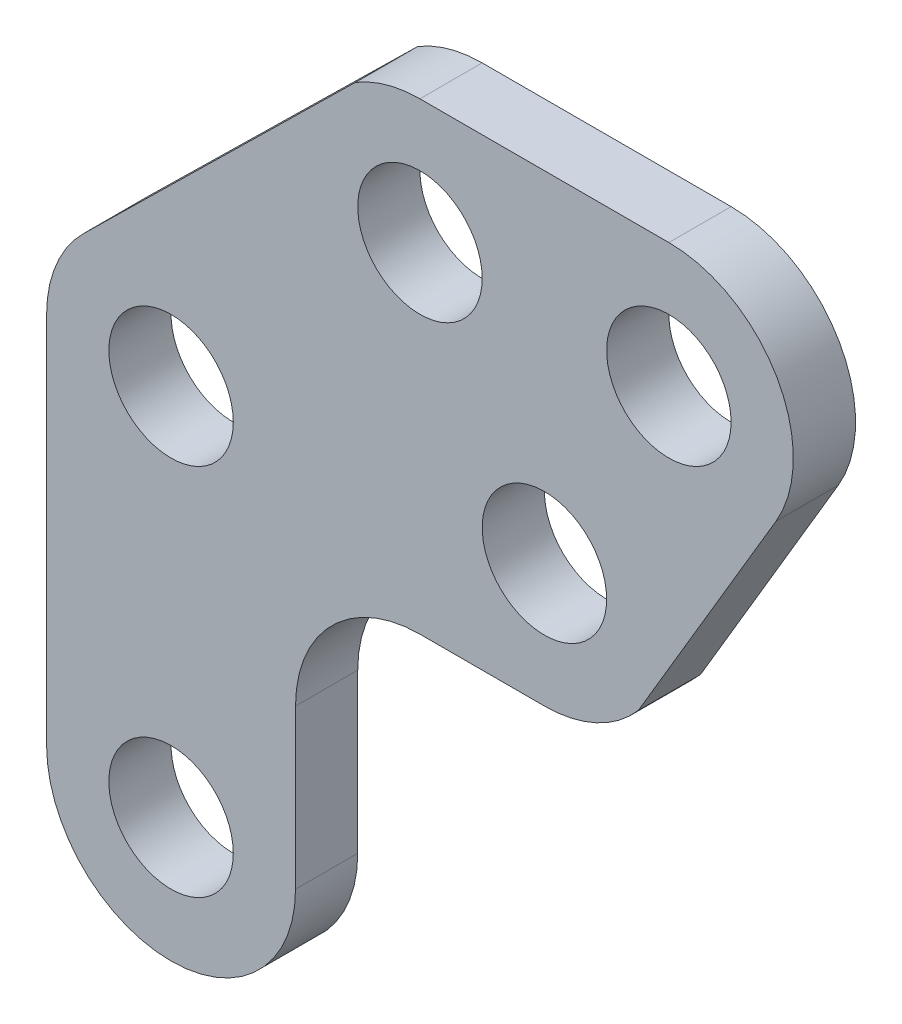
ISO-10303-21;
HEADER;
FILE_DESCRIPTION(('STEP AP214'),'2;1');
FILE_NAME('part.step','',(''),(''),'','','');
FILE_SCHEMA(('AUTOMOTIVE_DESIGN { 1 0 10303 214 1 1 1 1 }'));
ENDSEC;
DATA;
#1=APPLICATION_CONTEXT('core data for automotive mechanical design processes');
#2=APPLICATION_PROTOCOL_DEFINITION('international standard','automotive_design',2000,#1);
#3=PRODUCT_CONTEXT('',#1,'mechanical');
#4=PRODUCT('Part','Part','',(#3));
#5=PRODUCT_RELATED_PRODUCT_CATEGORY('part','',(#4));
#6=PRODUCT_DEFINITION_FORMATION('','',#4);
#7=PRODUCT_DEFINITION_CONTEXT('part definition',#1,'design');
#8=PRODUCT_DEFINITION('design','',#6,#7);
#9=PRODUCT_DEFINITION_SHAPE('','',#8);
#10=(LENGTH_UNIT() NAMED_UNIT(*) SI_UNIT(.MILLI.,.METRE.));
#11=(NAMED_UNIT(*) PLANE_ANGLE_UNIT() SI_UNIT($,.RADIAN.));
#12=(NAMED_UNIT(*) SI_UNIT($,.STERADIAN.) SOLID_ANGLE_UNIT());
#13=UNCERTAINTY_MEASURE_WITH_UNIT(LENGTH_MEASURE(1.E-05),#10,'distance_accuracy_value','');
#14=(GEOMETRIC_REPRESENTATION_CONTEXT(3) GLOBAL_UNCERTAINTY_ASSIGNED_CONTEXT((#13)) GLOBAL_UNIT_ASSIGNED_CONTEXT((#10,
#11,#12)) REPRESENTATION_CONTEXT('',''));
#15=CARTESIAN_POINT('',(0.,0.,0.));
#16=DIRECTION('',(0.,0.,1.));
#17=DIRECTION('',(1.,0.,0.));
#18=AXIS2_PLACEMENT_3D('',#15,#16,#17);
#19=CARTESIAN_POINT('',(0.,12.7,-3.175));
#20=DIRECTION('',(0.,0.,1.));
#21=DIRECTION('',(1.,0.,0.));
#22=AXIS2_PLACEMENT_3D('',#19,#20,#21);
#23=CYLINDRICAL_SURFACE('',#22,6.35);
#24=CARTESIAN_POINT('',(0.,12.7,0.));
#25=DIRECTION('',(0.,0.,1.));
#26=DIRECTION('',(1.,0.,0.));
#27=AXIS2_PLACEMENT_3D('',#24,#25,#26);
#28=CIRCLE('',#27,6.35);
#29=CARTESIAN_POINT('',(0.,19.05,0.));
#30=VERTEX_POINT('',#29);
#31=CARTESIAN_POINT('',(-3.29150229370883,18.1303326463956,0.));
#32=VERTEX_POINT('',#31);
#33=EDGE_CURVE('E163',#30,#32,#28,.T.);
#34=ORIENTED_EDGE('',*,*,#33,.F.);
#35=DIRECTION('',(0.,0.,1.));
#36=VECTOR('',#35,1.);
#37=CARTESIAN_POINT('',(0.,19.05,-3.175));
#38=LINE('',#37,#36);
#39=CARTESIAN_POINT('',(0.,19.05,-3.175));
#40=VERTEX_POINT('',#39);
#41=EDGE_CURVE('E11',#40,#30,#38,.T.);
#42=ORIENTED_EDGE('',*,*,#41,.F.);
#43=CARTESIAN_POINT('',(0.,12.7,-3.175));
#44=DIRECTION('',(0.,0.,1.));
#45=DIRECTION('',(1.,0.,0.));
#46=AXIS2_PLACEMENT_3D('',#43,#44,#45);
#47=CIRCLE('',#46,6.35);
#48=CARTESIAN_POINT('',(-3.29150229370883,18.1303326463956,-3.175));
#49=VERTEX_POINT('',#48);
#50=EDGE_CURVE('E197',#40,#49,#47,.T.);
#51=ORIENTED_EDGE('',*,*,#50,.T.);
#52=DIRECTION('',(0.,0.,1.));
#53=VECTOR('',#52,1.);
#54=CARTESIAN_POINT('',(-3.29150229370883,18.1303326463956,-3.175));
#55=LINE('',#54,#53);
#56=EDGE_CURVE('E46',#49,#32,#55,.T.);
#57=ORIENTED_EDGE('',*,*,#56,.T.);
#58=EDGE_LOOP('',(#34,#42,#51,#57));
#59=FACE_BOUND('',#58,.T.);
#60=ADVANCED_FACE('F43',(#59),#23,.T.);
#61=CARTESIAN_POINT('',(0.,19.05,-3.175));
#62=DIRECTION('',(0.,1.,0.));
#63=DIRECTION('',(0.,0.,1.));
#64=AXIS2_PLACEMENT_3D('',#61,#62,#63);
#65=PLANE('',#64);
#66=DIRECTION('',(-1.,0.,0.));
#67=VECTOR('',#66,1.);
#68=CARTESIAN_POINT('',(0.,19.05,0.));
#69=LINE('',#68,#67);
#70=CARTESIAN_POINT('',(12.7,19.05,0.));
#71=VERTEX_POINT('',#70);
#72=EDGE_CURVE('E191',#71,#30,#69,.T.);
#73=ORIENTED_EDGE('',*,*,#72,.F.);
#74=DIRECTION('',(0.,0.,1.));
#75=VECTOR('',#74,1.);
#76=CARTESIAN_POINT('',(12.7,19.05,-3.175));
#77=LINE('',#76,#75);
#78=CARTESIAN_POINT('',(12.7,19.05,-3.175));
#79=VERTEX_POINT('',#78);
#80=EDGE_CURVE('E55',#79,#71,#77,.T.);
#81=ORIENTED_EDGE('',*,*,#80,.F.);
#82=DIRECTION('',(-1.,0.,0.));
#83=VECTOR('',#82,1.);
#84=CARTESIAN_POINT('',(0.,19.05,-3.175));
#85=LINE('',#84,#83);
#86=EDGE_CURVE('E152',#79,#40,#85,.T.);
#87=ORIENTED_EDGE('',*,*,#86,.T.);
#88=ORIENTED_EDGE('',*,*,#41,.T.);
#89=EDGE_LOOP('',(#73,#81,#87,#88));
#90=FACE_BOUND('',#89,.T.);
#91=ADVANCED_FACE('F220',(#90),#65,.T.);
#92=CARTESIAN_POINT('',(12.7,12.7,-3.175));
#93=DIRECTION('',(0.,0.,1.));
#94=DIRECTION('',(1.,0.,0.));
#95=AXIS2_PLACEMENT_3D('',#92,#93,#94);
#96=CYLINDRICAL_SURFACE('',#95,6.35);
#97=CARTESIAN_POINT('',(12.7,12.7,0.));
#98=DIRECTION('',(0.,0.,1.));
#99=DIRECTION('',(1.,0.,0.));
#100=AXIS2_PLACEMENT_3D('',#97,#98,#99);
#101=CIRCLE('',#100,6.35);
#102=CARTESIAN_POINT('',(18.1648692173738,9.46616258340034,0.));
#103=VERTEX_POINT('',#102);
#104=EDGE_CURVE('E143',#103,#71,#101,.T.);
#105=ORIENTED_EDGE('',*,*,#104,.F.);
#106=DIRECTION('',(0.,0.,1.));
#107=VECTOR('',#106,1.);
#108=CARTESIAN_POINT('',(18.1648692173738,9.46616258340034,-3.175));
#109=LINE('',#108,#107);
#110=CARTESIAN_POINT('',(18.1648692173738,9.46616258340034,-3.175));
#111=VERTEX_POINT('',#110);
#112=EDGE_CURVE('E137',#111,#103,#109,.T.);
#113=ORIENTED_EDGE('',*,*,#112,.F.);
#114=CARTESIAN_POINT('',(12.7,12.7,-3.175));
#115=DIRECTION('',(0.,0.,1.));
#116=DIRECTION('',(1.,0.,0.));
#117=AXIS2_PLACEMENT_3D('',#114,#115,#116);
#118=CIRCLE('',#117,6.35);
#119=EDGE_CURVE('E139',#111,#79,#118,.T.);
#120=ORIENTED_EDGE('',*,*,#119,.T.);
#121=ORIENTED_EDGE('',*,*,#80,.T.);
#122=EDGE_LOOP('',(#105,#113,#120,#121));
#123=FACE_BOUND('',#122,.T.);
#124=ADVANCED_FACE('F138',(#123),#96,.T.);
#125=CARTESIAN_POINT('',(11.1439713813353,-2.39846866415228,-3.175));
#126=DIRECTION('',(0.86060932557068,-0.509265734897587,0.));
#127=DIRECTION('',(0.509265734897587,0.86060932557068,0.));
#128=AXIS2_PLACEMENT_3D('',#125,#126,#127);
#129=PLANE('',#128);
#130=DIRECTION('',(0.509265734897587,0.86060932557068,0.));
#131=VECTOR('',#130,1.);
#132=CARTESIAN_POINT('',(11.1439713813353,-2.39846866415228,0.));
#133=LINE('',#132,#131);
#134=CARTESIAN_POINT('',(11.1439713813353,-2.39846866415228,0.));
#135=VERTEX_POINT('',#134);
#136=EDGE_CURVE('E195',#135,#103,#133,.T.);
#137=ORIENTED_EDGE('',*,*,#136,.F.);
#138=DIRECTION('',(0.,0.,1.));
#139=VECTOR('',#138,1.);
#140=CARTESIAN_POINT('',(11.1439713813353,-2.39846866415228,-3.175));
#141=LINE('',#140,#139);
#142=CARTESIAN_POINT('',(11.1439713813353,-2.39846866415228,-3.175));
#143=VERTEX_POINT('',#142);
#144=EDGE_CURVE('E148',#143,#135,#141,.T.);
#145=ORIENTED_EDGE('',*,*,#144,.F.);
#146=DIRECTION('',(0.509265734897587,0.86060932557068,0.));
#147=VECTOR('',#146,1.);
#148=CARTESIAN_POINT('',(11.1439713813353,-2.39846866415228,-3.175));
#149=LINE('',#148,#147);
#150=EDGE_CURVE('E155',#143,#111,#149,.T.);
#151=ORIENTED_EDGE('',*,*,#150,.T.);
#152=ORIENTED_EDGE('',*,*,#112,.T.);
#153=EDGE_LOOP('',(#137,#145,#151,#152));
#154=FACE_BOUND('',#153,.T.);
#155=ADVANCED_FACE('F156',(#154),#129,.T.);
#156=CARTESIAN_POINT('',(6.34999999999995,1.70147737193766,-3.175));
#157=DIRECTION('',(0.,0.,1.));
#158=DIRECTION('',(1.,0.,0.));
#159=AXIS2_PLACEMENT_3D('',#156,#157,#158);
#160=CYLINDRICAL_SURFACE('',#159,6.30806777895673);
#161=CARTESIAN_POINT('',(6.34999999999995,1.70147737193766,0.));
#162=DIRECTION('',(0.,0.,1.));
#163=DIRECTION('',(1.,0.,0.));
#164=AXIS2_PLACEMENT_3D('',#161,#162,#163);
#165=CIRCLE('',#164,6.30806777895673);
#166=CARTESIAN_POINT('',(6.34999999999995,-4.60659040701907,0.));
#167=VERTEX_POINT('',#166);
#168=EDGE_CURVE('E188',#167,#135,#165,.T.);
#169=ORIENTED_EDGE('',*,*,#168,.F.);
#170=DIRECTION('',(0.,0.,1.));
#171=VECTOR('',#170,1.);
#172=CARTESIAN_POINT('',(6.34999999999995,-4.60659040701907,-3.175));
#173=LINE('',#172,#171);
#174=CARTESIAN_POINT('',(6.34999999999995,-4.60659040701907,-3.175));
#175=VERTEX_POINT('',#174);
#176=EDGE_CURVE('E203',#175,#167,#173,.T.);
#177=ORIENTED_EDGE('',*,*,#176,.F.);
#178=CARTESIAN_POINT('',(6.34999999999995,1.70147737193766,-3.175));
#179=DIRECTION('',(0.,0.,1.));
#180=DIRECTION('',(1.,0.,0.));
#181=AXIS2_PLACEMENT_3D('',#178,#179,#180);
#182=CIRCLE('',#181,6.30806777895673);
#183=EDGE_CURVE('E160',#175,#143,#182,.T.);
#184=ORIENTED_EDGE('',*,*,#183,.T.);
#185=ORIENTED_EDGE('',*,*,#144,.T.);
#186=EDGE_LOOP('',(#169,#177,#184,#185));
#187=FACE_BOUND('',#186,.T.);
#188=ADVANCED_FACE('F229',(#187),#160,.T.);
#189=CARTESIAN_POINT('',(6.34999999999995,-4.60659040701907,-3.175));
#190=DIRECTION('',(0.,-1.,0.));
#191=DIRECTION('',(1.,0.,0.));
#192=AXIS2_PLACEMENT_3D('',#189,#190,#191);
#193=PLANE('',#192);
#194=DIRECTION('',(1.,0.,0.));
#195=VECTOR('',#194,1.);
#196=CARTESIAN_POINT('',(6.34999999999995,-4.60659040701907,0.));
#197=LINE('',#196,#195);
#198=CARTESIAN_POINT('',(0.,-4.60659040701907,0.));
#199=VERTEX_POINT('',#198);
#200=EDGE_CURVE('E189',#199,#167,#197,.T.);
#201=ORIENTED_EDGE('',*,*,#200,.F.);
#202=DIRECTION('',(0.,0.,1.));
#203=VECTOR('',#202,1.);
#204=CARTESIAN_POINT('',(0.,-4.60659040701907,-3.175));
#205=LINE('',#204,#203);
#206=CARTESIAN_POINT('',(0.,-4.60659040701907,-3.175));
#207=VERTEX_POINT('',#206);
#208=EDGE_CURVE('E201',#207,#199,#205,.T.);
#209=ORIENTED_EDGE('',*,*,#208,.F.);
#210=DIRECTION('',(1.,0.,0.));
#211=VECTOR('',#210,1.);
#212=CARTESIAN_POINT('',(6.34999999999995,-4.60659040701907,-3.175));
#213=LINE('',#212,#211);
#214=EDGE_CURVE('E157',#207,#175,#213,.T.);
#215=ORIENTED_EDGE('',*,*,#214,.T.);
#216=ORIENTED_EDGE('',*,*,#176,.T.);
#217=EDGE_LOOP('',(#201,#209,#215,#216));
#218=FACE_BOUND('',#217,.T.);
#219=ADVANCED_FACE('F233',(#218),#193,.T.);
#220=CARTESIAN_POINT('',(0.,-10.9565904070191,-3.175));
#221=DIRECTION('',(0.,0.,1.));
#222=DIRECTION('',(1.,0.,0.));
#223=AXIS2_PLACEMENT_3D('',#220,#221,#222);
#224=CYLINDRICAL_SURFACE('',#223,6.34999999999999);
#225=CARTESIAN_POINT('',(0.,-10.9565904070191,0.));
#226=DIRECTION('',(0.,0.,-1.));
#227=DIRECTION('',(1.,0.,0.));
#228=AXIS2_PLACEMENT_3D('',#225,#226,#227);
#229=CIRCLE('',#228,6.34999999999999);
#230=CARTESIAN_POINT('',(-6.34999999999999,-10.9565904070191,0.));
#231=VERTEX_POINT('',#230);
#232=EDGE_CURVE('E181',#231,#199,#229,.T.);
#233=ORIENTED_EDGE('',*,*,#232,.F.);
#234=DIRECTION('',(0.,0.,1.));
#235=VECTOR('',#234,1.);
#236=CARTESIAN_POINT('',(-6.34999999999999,-10.9565904070191,-3.175));
#237=LINE('',#236,#235);
#238=CARTESIAN_POINT('',(-6.34999999999999,-10.9565904070191,-3.175));
#239=VERTEX_POINT('',#238);
#240=EDGE_CURVE('E202',#239,#231,#237,.T.);
#241=ORIENTED_EDGE('',*,*,#240,.F.);
#242=CARTESIAN_POINT('',(0.,-10.9565904070191,-3.175));
#243=DIRECTION('',(0.,0.,-1.));
#244=DIRECTION('',(1.,0.,0.));
#245=AXIS2_PLACEMENT_3D('',#242,#243,#244);
#246=CIRCLE('',#245,6.34999999999999);
#247=EDGE_CURVE('E340',#239,#207,#246,.T.);
#248=ORIENTED_EDGE('',*,*,#247,.T.);
#249=ORIENTED_EDGE('',*,*,#208,.T.);
#250=EDGE_LOOP('',(#233,#241,#248,#249));
#251=FACE_BOUND('',#250,.T.);
#252=ADVANCED_FACE('F240',(#251),#224,.F.);
#253=CARTESIAN_POINT('',(-6.34999999999999,-19.05,-3.175));
#254=DIRECTION('',(1.,0.,0.));
#255=DIRECTION('',(0.,0.,-1.));
#256=AXIS2_PLACEMENT_3D('',#253,#254,#255);
#257=PLANE('',#256);
#258=DIRECTION('',(0.,1.,0.));
#259=VECTOR('',#258,1.);
#260=CARTESIAN_POINT('',(-6.34999999999999,-19.05,0.));
#261=LINE('',#260,#259);
#262=CARTESIAN_POINT('',(-6.34999999999999,-19.05,0.));
#263=VERTEX_POINT('',#262);
#264=EDGE_CURVE('E179',#263,#231,#261,.T.);
#265=ORIENTED_EDGE('',*,*,#264,.F.);
#266=DIRECTION('',(0.,0.,1.));
#267=VECTOR('',#266,1.);
#268=CARTESIAN_POINT('',(-6.34999999999999,-19.05,-3.175));
#269=LINE('',#268,#267);
#270=CARTESIAN_POINT('',(-6.34999999999999,-19.05,-3.175));
#271=VERTEX_POINT('',#270);
#272=EDGE_CURVE('E210',#271,#263,#269,.T.);
#273=ORIENTED_EDGE('',*,*,#272,.F.);
#274=DIRECTION('',(0.,1.,0.));
#275=VECTOR('',#274,1.);
#276=CARTESIAN_POINT('',(-6.34999999999999,-19.05,-3.175));
#277=LINE('',#276,#275);
#278=EDGE_CURVE('E331',#271,#239,#277,.T.);
#279=ORIENTED_EDGE('',*,*,#278,.T.);
#280=ORIENTED_EDGE('',*,*,#240,.T.);
#281=EDGE_LOOP('',(#265,#273,#279,#280));
#282=FACE_BOUND('',#281,.T.);
#283=ADVANCED_FACE('F244',(#282),#257,.T.);
#284=CARTESIAN_POINT('',(-12.7,-19.05,-3.175));
#285=DIRECTION('',(0.,0.,1.));
#286=DIRECTION('',(1.,0.,0.));
#287=AXIS2_PLACEMENT_3D('',#284,#285,#286);
#288=CYLINDRICAL_SURFACE('',#287,6.35);
#289=CARTESIAN_POINT('',(-12.7,-19.05,0.));
#290=DIRECTION('',(0.,0.,1.));
#291=DIRECTION('',(1.,0.,0.));
#292=AXIS2_PLACEMENT_3D('',#289,#290,#291);
#293=CIRCLE('',#292,6.35);
#294=CARTESIAN_POINT('',(-19.05,-19.05,0.));
#295=VERTEX_POINT('',#294);
#296=EDGE_CURVE('E180',#295,#263,#293,.T.);
#297=ORIENTED_EDGE('',*,*,#296,.F.);
#298=DIRECTION('',(0.,0.,1.));
#299=VECTOR('',#298,1.);
#300=CARTESIAN_POINT('',(-19.05,-19.05,-3.175));
#301=LINE('',#300,#299);
#302=CARTESIAN_POINT('',(-19.05,-19.05,-3.175));
#303=VERTEX_POINT('',#302);
#304=EDGE_CURVE('E207',#303,#295,#301,.T.);
#305=ORIENTED_EDGE('',*,*,#304,.F.);
#306=CARTESIAN_POINT('',(-12.7,-19.05,-3.175));
#307=DIRECTION('',(0.,0.,1.));
#308=DIRECTION('',(1.,0.,0.));
#309=AXIS2_PLACEMENT_3D('',#306,#307,#308);
#310=CIRCLE('',#309,6.35);
#311=EDGE_CURVE('E332',#303,#271,#310,.T.);
#312=ORIENTED_EDGE('',*,*,#311,.T.);
#313=ORIENTED_EDGE('',*,*,#272,.T.);
#314=EDGE_LOOP('',(#297,#305,#312,#313));
#315=FACE_BOUND('',#314,.T.);
#316=ADVANCED_FACE('F242',(#315),#288,.T.);
#317=CARTESIAN_POINT('',(-19.05,-19.05,-3.175));
#318=DIRECTION('',(-1.,0.,0.));
#319=DIRECTION('',(0.,-1.,0.));
#320=AXIS2_PLACEMENT_3D('',#317,#318,#319);
#321=PLANE('',#320);
#322=DIRECTION('',(0.,-1.,0.));
#323=VECTOR('',#322,1.);
#324=CARTESIAN_POINT('',(-19.05,-19.05,0.));
#325=LINE('',#324,#323);
#326=CARTESIAN_POINT('',(-19.05,0.,0.));
#327=VERTEX_POINT('',#326);
#328=EDGE_CURVE('E173',#327,#295,#325,.T.);
#329=ORIENTED_EDGE('',*,*,#328,.F.);
#330=DIRECTION('',(0.,0.,1.));
#331=VECTOR('',#330,1.);
#332=CARTESIAN_POINT('',(-19.05,0.,-3.175));
#333=LINE('',#332,#331);
#334=CARTESIAN_POINT('',(-19.05,0.,-3.175));
#335=VERTEX_POINT('',#334);
#336=EDGE_CURVE('E211',#335,#327,#333,.T.);
#337=ORIENTED_EDGE('',*,*,#336,.F.);
#338=DIRECTION('',(0.,-1.,0.));
#339=VECTOR('',#338,1.);
#340=CARTESIAN_POINT('',(-19.05,-19.05,-3.175));
#341=LINE('',#340,#339);
#342=EDGE_CURVE('E327',#335,#303,#341,.T.);
#343=ORIENTED_EDGE('',*,*,#342,.T.);
#344=ORIENTED_EDGE('',*,*,#304,.T.);
#345=EDGE_LOOP('',(#329,#337,#343,#344));
#346=FACE_BOUND('',#345,.T.);
#347=ADVANCED_FACE('F249',(#346),#321,.T.);
#348=CARTESIAN_POINT('',(-12.7,0.,-3.175));
#349=DIRECTION('',(0.,0.,1.));
#350=DIRECTION('',(1.,0.,0.));
#351=AXIS2_PLACEMENT_3D('',#348,#349,#350);
#352=CYLINDRICAL_SURFACE('',#351,6.35);
#353=CARTESIAN_POINT('',(-12.7,0.,0.));
#354=DIRECTION('',(0.,0.,1.));
#355=DIRECTION('',(1.,0.,0.));
#356=AXIS2_PLACEMENT_3D('',#353,#354,#355);
#357=CIRCLE('',#356,6.35);
#358=CARTESIAN_POINT('',(-17.1477321327365,4.53212741164928,0.));
#359=VERTEX_POINT('',#358);
#360=EDGE_CURVE('E171',#359,#327,#357,.T.);
#361=ORIENTED_EDGE('',*,*,#360,.F.);
#362=DIRECTION('',(0.,0.,1.));
#363=VECTOR('',#362,1.);
#364=CARTESIAN_POINT('',(-17.1477321327365,4.53212741164928,-3.175));
#365=LINE('',#364,#363);
#366=CARTESIAN_POINT('',(-17.1477321327365,4.53212741164928,-3.175));
#367=VERTEX_POINT('',#366);
#368=EDGE_CURVE('E215',#367,#359,#365,.T.);
#369=ORIENTED_EDGE('',*,*,#368,.F.);
#370=CARTESIAN_POINT('',(-12.7,0.,-3.175));
#371=DIRECTION('',(0.,0.,1.));
#372=DIRECTION('',(1.,0.,0.));
#373=AXIS2_PLACEMENT_3D('',#370,#371,#372);
#374=CIRCLE('',#373,6.35);
#375=EDGE_CURVE('E324',#367,#335,#374,.T.);
#376=ORIENTED_EDGE('',*,*,#375,.T.);
#377=ORIENTED_EDGE('',*,*,#336,.T.);
#378=EDGE_LOOP('',(#361,#369,#376,#377));
#379=FACE_BOUND('',#378,.T.);
#380=ADVANCED_FACE('F251',(#379),#352,.T.);
#381=CARTESIAN_POINT('',(-17.1477321327365,4.53212741164928,-3.175));
#382=DIRECTION('',(-0.700430257123865,0.713720852228234,0.));
#383=DIRECTION('',(-0.713720852228234,-0.700430257123865,0.));
#384=AXIS2_PLACEMENT_3D('',#381,#382,#383);
#385=PLANE('',#384);
#386=DIRECTION('',(-0.713720852228234,-0.700430257123865,0.));
#387=VECTOR('',#386,1.);
#388=CARTESIAN_POINT('',(-17.1477321327365,4.53212741164928,0.));
#389=LINE('',#388,#387);
#390=EDGE_CURVE('E170',#32,#359,#389,.T.);
#391=ORIENTED_EDGE('',*,*,#390,.F.);
#392=ORIENTED_EDGE('',*,*,#56,.F.);
#393=DIRECTION('',(-0.713720852228234,-0.700430257123865,0.));
#394=VECTOR('',#393,1.);
#395=CARTESIAN_POINT('',(-17.1477321327365,4.53212741164928,-3.175));
#396=LINE('',#395,#394);
#397=EDGE_CURVE('E323',#49,#367,#396,.T.);
#398=ORIENTED_EDGE('',*,*,#397,.T.);
#399=ORIENTED_EDGE('',*,*,#368,.T.);
#400=EDGE_LOOP('',(#391,#392,#398,#399));
#401=FACE_BOUND('',#400,.T.);
#402=ADVANCED_FACE('F212',(#401),#385,.T.);
#403=CARTESIAN_POINT('',(0.,12.7,-3.175));
#404=DIRECTION('',(0.,0.,1.));
#405=DIRECTION('',(1.,0.,0.));
#406=AXIS2_PLACEMENT_3D('',#403,#404,#405);
#407=PLANE('',#406);
#408=CARTESIAN_POINT('',(12.7,12.7,-3.175));
#409=DIRECTION('',(0.,0.,1.));
#410=DIRECTION('',(1.,0.,0.));
#411=AXIS2_PLACEMENT_3D('',#408,#409,#410);
#412=CIRCLE('',#411,3.175);
#413=CARTESIAN_POINT('',(15.875,12.7,-3.175));
#414=VERTEX_POINT('',#413);
#415=EDGE_CURVE('E295',#414,#414,#412,.T.);
#416=ORIENTED_EDGE('',*,*,#415,.T.);
#417=EDGE_LOOP('',(#416));
#418=FACE_BOUND('',#417,.T.);
#419=CARTESIAN_POINT('',(0.,12.7,-3.175));
#420=DIRECTION('',(0.,0.,1.));
#421=DIRECTION('',(1.,0.,0.));
#422=AXIS2_PLACEMENT_3D('',#419,#420,#421);
#423=CIRCLE('',#422,3.175);
#424=CARTESIAN_POINT('',(3.175,12.7,-3.175));
#425=VERTEX_POINT('',#424);
#426=EDGE_CURVE('E297',#425,#425,#423,.T.);
#427=ORIENTED_EDGE('',*,*,#426,.T.);
#428=EDGE_LOOP('',(#427));
#429=FACE_BOUND('',#428,.T.);
#430=CARTESIAN_POINT('',(6.34999999999995,1.70147737193766,-3.175));
#431=DIRECTION('',(0.,0.,1.));
#432=DIRECTION('',(1.,0.,0.));
#433=AXIS2_PLACEMENT_3D('',#430,#431,#432);
#434=CIRCLE('',#433,3.175);
#435=CARTESIAN_POINT('',(9.52499999999995,1.70147737193766,-3.175));
#436=VERTEX_POINT('',#435);
#437=EDGE_CURVE('E308',#436,#436,#434,.T.);
#438=ORIENTED_EDGE('',*,*,#437,.T.);
#439=EDGE_LOOP('',(#438));
#440=FACE_BOUND('',#439,.T.);
#441=CARTESIAN_POINT('',(-12.7,-19.05,-3.175));
#442=DIRECTION('',(0.,0.,1.));
#443=DIRECTION('',(1.,0.,0.));
#444=AXIS2_PLACEMENT_3D('',#441,#442,#443);
#445=CIRCLE('',#444,3.175);
#446=CARTESIAN_POINT('',(-9.52499999999999,-19.05,-3.175));
#447=VERTEX_POINT('',#446);
#448=EDGE_CURVE('E315',#447,#447,#445,.T.);
#449=ORIENTED_EDGE('',*,*,#448,.T.);
#450=EDGE_LOOP('',(#449));
#451=FACE_BOUND('',#450,.T.);
#452=CARTESIAN_POINT('',(-12.7,0.,-3.175));
#453=DIRECTION('',(0.,0.,1.));
#454=DIRECTION('',(1.,0.,0.));
#455=AXIS2_PLACEMENT_3D('',#452,#453,#454);
#456=CIRCLE('',#455,3.175);
#457=CARTESIAN_POINT('',(-9.52499999999999,0.,-3.175));
#458=VERTEX_POINT('',#457);
#459=EDGE_CURVE('E169',#458,#458,#456,.T.);
#460=ORIENTED_EDGE('',*,*,#459,.T.);
#461=EDGE_LOOP('',(#460));
#462=FACE_BOUND('',#461,.T.);
#463=ORIENTED_EDGE('',*,*,#50,.F.);
#464=ORIENTED_EDGE('',*,*,#86,.F.);
#465=ORIENTED_EDGE('',*,*,#119,.F.);
#466=ORIENTED_EDGE('',*,*,#150,.F.);
#467=ORIENTED_EDGE('',*,*,#183,.F.);
#468=ORIENTED_EDGE('',*,*,#214,.F.);
#469=ORIENTED_EDGE('',*,*,#247,.F.);
#470=ORIENTED_EDGE('',*,*,#278,.F.);
#471=ORIENTED_EDGE('',*,*,#311,.F.);
#472=ORIENTED_EDGE('',*,*,#342,.F.);
#473=ORIENTED_EDGE('',*,*,#375,.F.);
#474=ORIENTED_EDGE('',*,*,#397,.F.);
#475=EDGE_LOOP('',(#463,#464,#465,#466,#467,#468,#469,#470,#471,#472,#473,#474));
#476=FACE_BOUND('',#475,.T.);
#477=ADVANCED_FACE('F147',(#418,#429,#440,#451,#462,#476),#407,.F.);
#478=CARTESIAN_POINT('',(0.,12.7,0.));
#479=DIRECTION('',(0.,0.,1.));
#480=DIRECTION('',(1.,0.,0.));
#481=AXIS2_PLACEMENT_3D('',#478,#479,#480);
#482=PLANE('',#481);
#483=CARTESIAN_POINT('',(12.7,12.7,0.));
#484=DIRECTION('',(0.,0.,1.));
#485=DIRECTION('',(1.,0.,0.));
#486=AXIS2_PLACEMENT_3D('',#483,#484,#485);
#487=CIRCLE('',#486,3.175);
#488=CARTESIAN_POINT('',(15.875,12.7,0.));
#489=VERTEX_POINT('',#488);
#490=EDGE_CURVE('E293',#489,#489,#487,.T.);
#491=ORIENTED_EDGE('',*,*,#490,.F.);
#492=EDGE_LOOP('',(#491));
#493=FACE_BOUND('',#492,.T.);
#494=CARTESIAN_POINT('',(0.,12.7,0.));
#495=DIRECTION('',(0.,0.,1.));
#496=DIRECTION('',(1.,0.,0.));
#497=AXIS2_PLACEMENT_3D('',#494,#495,#496);
#498=CIRCLE('',#497,3.175);
#499=CARTESIAN_POINT('',(3.175,12.7,0.));
#500=VERTEX_POINT('',#499);
#501=EDGE_CURVE('E296',#500,#500,#498,.T.);
#502=ORIENTED_EDGE('',*,*,#501,.F.);
#503=EDGE_LOOP('',(#502));
#504=FACE_BOUND('',#503,.T.);
#505=CARTESIAN_POINT('',(6.34999999999995,1.70147737193766,0.));
#506=DIRECTION('',(0.,0.,1.));
#507=DIRECTION('',(1.,0.,0.));
#508=AXIS2_PLACEMENT_3D('',#505,#506,#507);
#509=CIRCLE('',#508,3.175);
#510=CARTESIAN_POINT('',(9.52499999999995,1.70147737193766,0.));
#511=VERTEX_POINT('',#510);
#512=EDGE_CURVE('E303',#511,#511,#509,.T.);
#513=ORIENTED_EDGE('',*,*,#512,.F.);
#514=EDGE_LOOP('',(#513));
#515=FACE_BOUND('',#514,.T.);
#516=CARTESIAN_POINT('',(-12.7,-19.05,0.));
#517=DIRECTION('',(0.,0.,1.));
#518=DIRECTION('',(1.,0.,0.));
#519=AXIS2_PLACEMENT_3D('',#516,#517,#518);
#520=CIRCLE('',#519,3.175);
#521=CARTESIAN_POINT('',(-9.52499999999999,-19.05,0.));
#522=VERTEX_POINT('',#521);
#523=EDGE_CURVE('E310',#522,#522,#520,.T.);
#524=ORIENTED_EDGE('',*,*,#523,.F.);
#525=EDGE_LOOP('',(#524));
#526=FACE_BOUND('',#525,.T.);
#527=CARTESIAN_POINT('',(-12.7,0.,0.));
#528=DIRECTION('',(0.,0.,1.));
#529=DIRECTION('',(1.,0.,0.));
#530=AXIS2_PLACEMENT_3D('',#527,#528,#529);
#531=CIRCLE('',#530,3.175);
#532=CARTESIAN_POINT('',(-9.52499999999999,0.,0.));
#533=VERTEX_POINT('',#532);
#534=EDGE_CURVE('E312',#533,#533,#531,.T.);
#535=ORIENTED_EDGE('',*,*,#534,.F.);
#536=EDGE_LOOP('',(#535));
#537=FACE_BOUND('',#536,.T.);
#538=ORIENTED_EDGE('',*,*,#33,.T.);
#539=ORIENTED_EDGE('',*,*,#390,.T.);
#540=ORIENTED_EDGE('',*,*,#360,.T.);
#541=ORIENTED_EDGE('',*,*,#328,.T.);
#542=ORIENTED_EDGE('',*,*,#296,.T.);
#543=ORIENTED_EDGE('',*,*,#264,.T.);
#544=ORIENTED_EDGE('',*,*,#232,.T.);
#545=ORIENTED_EDGE('',*,*,#200,.T.);
#546=ORIENTED_EDGE('',*,*,#168,.T.);
#547=ORIENTED_EDGE('',*,*,#136,.T.);
#548=ORIENTED_EDGE('',*,*,#104,.T.);
#549=ORIENTED_EDGE('',*,*,#72,.T.);
#550=EDGE_LOOP('',(#538,#539,#540,#541,#542,#543,#544,#545,#546,#547,#548,#549));
#551=FACE_BOUND('',#550,.T.);
#552=ADVANCED_FACE('F216',(#493,#504,#515,#526,#537,#551),#482,.T.);
#553=CARTESIAN_POINT('',(-12.7,0.,-3.175));
#554=DIRECTION('',(0.,0.,1.));
#555=DIRECTION('',(1.,0.,0.));
#556=AXIS2_PLACEMENT_3D('',#553,#554,#555);
#557=CYLINDRICAL_SURFACE('',#556,3.175);
#558=ORIENTED_EDGE('',*,*,#459,.F.);
#559=EDGE_LOOP('',(#558));
#560=FACE_BOUND('',#559,.T.);
#561=ORIENTED_EDGE('',*,*,#534,.T.);
#562=EDGE_LOOP('',(#561));
#563=FACE_BOUND('',#562,.T.);
#564=ADVANCED_FACE('F264',(#560,#563),#557,.F.);
#565=CARTESIAN_POINT('',(-12.7,-19.05,-3.175));
#566=DIRECTION('',(0.,0.,1.));
#567=DIRECTION('',(1.,0.,0.));
#568=AXIS2_PLACEMENT_3D('',#565,#566,#567);
#569=CYLINDRICAL_SURFACE('',#568,3.175);
#570=ORIENTED_EDGE('',*,*,#448,.F.);
#571=EDGE_LOOP('',(#570));
#572=FACE_BOUND('',#571,.T.);
#573=ORIENTED_EDGE('',*,*,#523,.T.);
#574=EDGE_LOOP('',(#573));
#575=FACE_BOUND('',#574,.T.);
#576=ADVANCED_FACE('F275',(#572,#575),#569,.F.);
#577=CARTESIAN_POINT('',(6.34999999999995,1.70147737193766,-3.175));
#578=DIRECTION('',(0.,0.,1.));
#579=DIRECTION('',(1.,0.,0.));
#580=AXIS2_PLACEMENT_3D('',#577,#578,#579);
#581=CYLINDRICAL_SURFACE('',#580,3.175);
#582=ORIENTED_EDGE('',*,*,#437,.F.);
#583=EDGE_LOOP('',(#582));
#584=FACE_BOUND('',#583,.T.);
#585=ORIENTED_EDGE('',*,*,#512,.T.);
#586=EDGE_LOOP('',(#585));
#587=FACE_BOUND('',#586,.T.);
#588=ADVANCED_FACE('F277',(#584,#587),#581,.F.);
#589=CARTESIAN_POINT('',(0.,12.7,-3.175));
#590=DIRECTION('',(0.,0.,1.));
#591=DIRECTION('',(1.,0.,0.));
#592=AXIS2_PLACEMENT_3D('',#589,#590,#591);
#593=CYLINDRICAL_SURFACE('',#592,3.175);
#594=ORIENTED_EDGE('',*,*,#426,.F.);
#595=EDGE_LOOP('',(#594));
#596=FACE_BOUND('',#595,.T.);
#597=ORIENTED_EDGE('',*,*,#501,.T.);
#598=EDGE_LOOP('',(#597));
#599=FACE_BOUND('',#598,.T.);
#600=ADVANCED_FACE('F278',(#596,#599),#593,.F.);
#601=CARTESIAN_POINT('',(12.7,12.7,-3.175));
#602=DIRECTION('',(0.,0.,1.));
#603=DIRECTION('',(1.,0.,0.));
#604=AXIS2_PLACEMENT_3D('',#601,#602,#603);
#605=CYLINDRICAL_SURFACE('',#604,3.175);
#606=ORIENTED_EDGE('',*,*,#415,.F.);
#607=EDGE_LOOP('',(#606));
#608=FACE_BOUND('',#607,.T.);
#609=ORIENTED_EDGE('',*,*,#490,.T.);
#610=EDGE_LOOP('',(#609));
#611=FACE_BOUND('',#610,.T.);
#612=ADVANCED_FACE('F283',(#608,#611),#605,.F.);
#613=CLOSED_SHELL('',(#60,#91,#124,#155,#188,#219,#252,#283,#316,#347,#380,#402,#477,#552,#564,
#576,#588,#600,#612));
#614=MANIFOLD_SOLID_BREP('B2',#613);
#615=ADVANCED_BREP_SHAPE_REPRESENTATION('',(#18,#614),#14);
#616=SHAPE_DEFINITION_REPRESENTATION(#9,#615);
ENDSEC;
END-ISO-10303-21;
